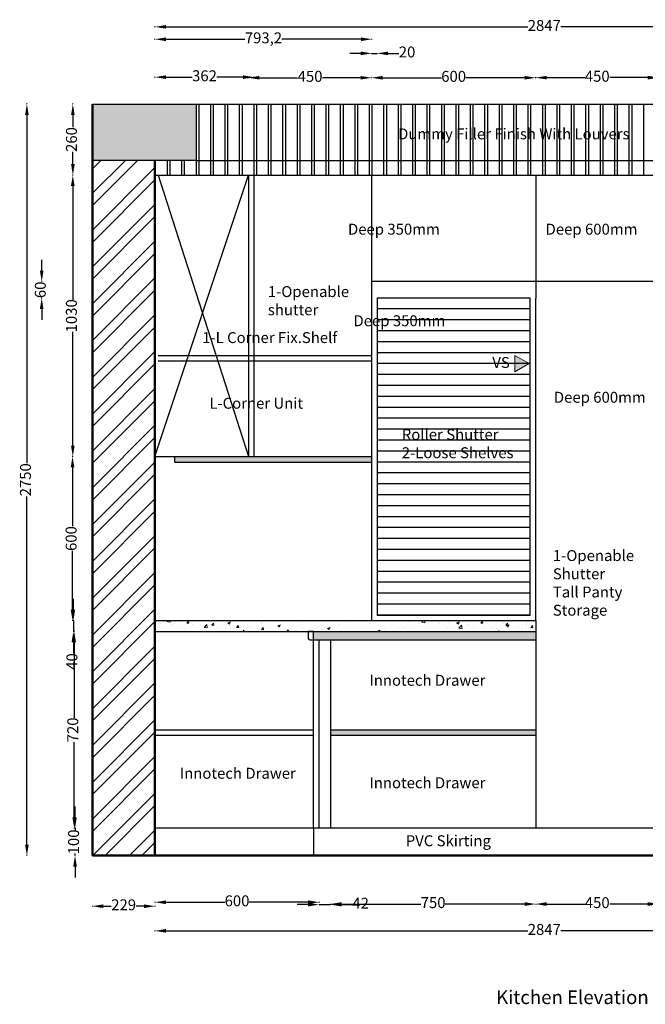
# Model space of a CAD drawing. Units: millimetres. Extents: x 2054 to 5837, y -782 to 2821.
# Tile 1 of 2: x 2054 to 4342, y -782 to 2821. Entities that reach past the tile are written whole.
import ezdxf

# ---------------------------------------------------------------- set-up
doc = ezdxf.new("R2010")
doc.units = ezdxf.units.MM
for name, color, linetype, lineweight in [('A-ANNO-DIMS', 2, 'Continuous', 18), ('A-ANNO-SYMB', 1, 'Continuous', 18), ('A-ANNO-TEXT', 7, 'Continuous', 18), ('A-FURN', 42, 'Continuous', 25), ('A-FURN-PATT', 8, 'Continuous', 13), ('A-WALL', 7, 'Continuous', 50), ('A-WALL-PATT', 8, 'Continuous', 13)]:
    doc.layers.add(name, color=color, linetype=linetype, lineweight=lineweight)
doc.styles.get("Standard").update_dxf_attribs({"font": 'arial.ttf'})
doc.dimstyles.new('ISO-25', dxfattribs={"dimtxt": 40, "dimasz": 40, "dimexe": 1.25, "dimexo": 0.625, "dimtad": 0, "dimtxsty": 'Standard', "dimcen": 2.5, "dimclrt": 1, "dimadec": 0, "dimazin": 0, "dimtfac": 1, "dimtmove": 0, "dimatfit": 3, "dimfxl": 1, "dimfxlon": 1, "dimarcsym": 0})

# ---------------------------------------------------------------- blocks, each defined once
blk = doc.blocks.new('*D2')
at = {"layer": 'A-ANNO-DIMS', "color": 0, "lineweight": -2, "transparency": 16777216}
for p, q in [((3941.1, -414.1), (3941.1, -416.4)), ((3981.1, -415.1), (4120.6, -415.1)), ((4351.1, -415.1), (4211.7, -415.1)), ((4391.1, -414.1), (4391.1, -416.4))]:
    blk.add_line(p, q, dxfattribs=at)
at = {"layer": 'A-ANNO-DIMS', "color": 0, "transparency": 16777216}
for points in [[(3981.1, -408.4), (3981.1, -421.8), (3941.1, -415.1)], [(4351.1, -408.4), (4351.1, -421.8), (4391.1, -415.1)]]:
    blk.add_solid(points, dxfattribs=at)
at = {"layer": 'Defpoints', "color": 0, "transparency": 16777216}
for p in [(3941.1, -137.8), (4391.1, -137.8), (3941.1, -415.1)]:
    blk.add_point(p, dxfattribs=at)
at = {"layer": 'A-ANNO-DIMS', "color": 0, "transparency": 16777216, "insert": (4166.1, -415.1), "char_height": 40, "attachment_point": 5}
blk.add_mtext('450', dxfattribs=at)
blk = doc.blocks.new('*D3')
at = {"layer": 'A-ANNO-DIMS', "color": 0, "lineweight": -2, "transparency": 16777216}
for p, q in [((3191.1, -414.1), (3191.1, -416.4)), ((3231.1, -415.1), (3521.5, -415.1)), ((3901.1, -415.1), (3610.7, -415.1)), ((3941.1, -414.1), (3941.1, -416.4))]:
    blk.add_line(p, q, dxfattribs=at)
at = {"layer": 'A-ANNO-DIMS', "color": 0, "transparency": 16777216}
for points in [[(3231.1, -408.4), (3231.1, -421.8), (3191.1, -415.1)], [(3901.1, -408.4), (3901.1, -421.8), (3941.1, -415.1)]]:
    blk.add_solid(points, dxfattribs=at)
at = {"layer": 'Defpoints', "color": 0, "transparency": 16777216}
for p in [(3191.1, -137.8), (3941.1, -137.8), (3191.1, -415.1)]:
    blk.add_point(p, dxfattribs=at)
at = {"layer": 'A-ANNO-DIMS', "color": 0, "transparency": 16777216, "insert": (3566.1, -415.1), "char_height": 40, "attachment_point": 5}
blk.add_mtext('750', dxfattribs=at)
blk = doc.blocks.new('*D4')
at = {"layer": 'A-ANNO-DIMS', "color": 0, "lineweight": -2, "transparency": 16777216}
for p, q in [((3109.1, -417.2), (3069.1, -417.2)), ((3149.1, -416.2), (3149.1, -418.5)), ((3149.1, -417.2), (3191.1, -417.2)), ((3191.1, -416.2), (3191.1, -418.5)), ((3231.1, -417.2), (3271.1, -417.2))]:
    blk.add_line(p, q, dxfattribs=at)
at = {"layer": 'A-ANNO-DIMS', "color": 0, "transparency": 16777216}
for points in [[(3109.1, -410.6), (3109.1, -423.9), (3149.1, -417.2)], [(3231.1, -410.6), (3231.1, -423.9), (3191.1, -417.2)]]:
    blk.add_solid(points, dxfattribs=at)
at = {"layer": 'Defpoints', "color": 0, "transparency": 16777216}
for p in [(3149.1, -137.8), (3191.1, -137.8), (3191.1, -417.2)]:
    blk.add_point(p, dxfattribs=at)
at = {"layer": 'A-ANNO-DIMS', "color": 0, "transparency": 16777216, "insert": (3301, -417.2), "char_height": 40, "attachment_point": 5}
blk.add_mtext('42', dxfattribs=at)
blk = doc.blocks.new('*D5')
at = {"layer": 'A-ANNO-DIMS', "color": 0, "lineweight": -2, "transparency": 16777216}
for p, q in [((2549.1, -407.6), (2549.1, -409.8)), ((2589.1, -408.6), (2804.3, -408.6)), ((3109.1, -408.6), (2894, -408.6)), ((3149.1, -407.6), (3149.1, -409.8))]:
    blk.add_line(p, q, dxfattribs=at)
at = {"layer": 'A-ANNO-DIMS', "color": 0, "transparency": 16777216}
for points in [[(2589.1, -401.9), (2589.1, -415.3), (2549.1, -408.6)], [(3109.1, -401.9), (3109.1, -415.3), (3149.1, -408.6)]]:
    blk.add_solid(points, dxfattribs=at)
at = {"layer": 'Defpoints', "color": 0, "transparency": 16777216}
for p in [(2549.1, -137.8), (3149.1, -137.8), (2549.1, -408.6)]:
    blk.add_point(p, dxfattribs=at)
at = {"layer": 'A-ANNO-DIMS', "color": 0, "transparency": 16777216, "insert": (2849.1, -408.6), "char_height": 40, "attachment_point": 5}
blk.add_mtext('600', dxfattribs=at)
blk = doc.blocks.new('*D6')
at = {"layer": 'A-ANNO-DIMS', "color": 0, "lineweight": -2, "transparency": 16777216}
for p, q in [((2549.1, -512.1), (2549.1, -514.3)), ((2589.1, -513.1), (3911.9, -513.1)), ((5356.1, -513.1), (4033.3, -513.1)), ((5396.1, -512.1), (5396.1, -514.3))]:
    blk.add_line(p, q, dxfattribs=at)
at = {"layer": 'A-ANNO-DIMS', "color": 0, "transparency": 16777216}
for points in [[(2589.1, -506.4), (2589.1, -519.7), (2549.1, -513.1)], [(5356.1, -506.4), (5356.1, -519.7), (5396.1, -513.1)]]:
    blk.add_solid(points, dxfattribs=at)
at = {"layer": 'Defpoints', "color": 0, "transparency": 16777216}
for p in [(2549.1, -237.8), (5396.1, -237.8), (5396.1, -513.1)]:
    blk.add_point(p, dxfattribs=at)
at = {"layer": 'A-ANNO-DIMS', "color": 0, "transparency": 16777216, "insert": (3972.6, -513.1), "char_height": 40, "attachment_point": 5}
blk.add_mtext('2847', dxfattribs=at)
blk = doc.blocks.new('*D13')
at = {"layer": 'A-ANNO-DIMS', "color": 0, "lineweight": -2, "transparency": 16777216}
for p, q in [((3941.1, 2607.6), (3941.1, 2609.9)), ((3981.1, 2608.6), (4120.6, 2608.6)), ((4351.1, 2608.6), (4211.7, 2608.6)), ((4391.1, 2607.6), (4391.1, 2609.9))]:
    blk.add_line(p, q, dxfattribs=at)
at = {"layer": 'A-ANNO-DIMS', "color": 0, "transparency": 16777216}
for points in [[(3981.1, 2615.3), (3981.1, 2602), (3941.1, 2608.6)], [(4351.1, 2615.3), (4351.1, 2602), (4391.1, 2608.6)]]:
    blk.add_solid(points, dxfattribs=at)
at = {"layer": 'Defpoints', "color": 0, "transparency": 16777216}
for p in [(3941.1, 2608.6), (3941.1, 2252.2), (4391.1, 2252.2)]:
    blk.add_point(p, dxfattribs=at)
at = {"layer": 'A-ANNO-DIMS', "color": 0, "transparency": 16777216, "insert": (4166.1, 2608.6), "char_height": 40, "attachment_point": 5}
blk.add_mtext('450', dxfattribs=at)
blk = doc.blocks.new('*D14')
at = {"layer": 'A-ANNO-DIMS', "color": 0, "lineweight": -2, "transparency": 16777216}
for p, q in [((3341.1, 2607.2), (3341.1, 2609.5)), ((3381.1, 2608.2), (3596.3, 2608.2)), ((3901.1, 2608.2), (3686, 2608.2)), ((3941.1, 2607.2), (3941.1, 2609.5))]:
    blk.add_line(p, q, dxfattribs=at)
at = {"layer": 'A-ANNO-DIMS', "color": 0, "transparency": 16777216}
for points in [[(3381.1, 2614.9), (3381.1, 2601.6), (3341.1, 2608.2)], [(3901.1, 2614.9), (3901.1, 2601.6), (3941.1, 2608.2)]]:
    blk.add_solid(points, dxfattribs=at)
at = {"layer": 'Defpoints', "color": 0, "transparency": 16777216}
for p in [(3341.1, 2608.2), (3341.1, 2252.2), (3941.1, 2252.2)]:
    blk.add_point(p, dxfattribs=at)
at = {"layer": 'A-ANNO-DIMS', "color": 0, "transparency": 16777216, "insert": (3641.1, 2608.2), "char_height": 40, "attachment_point": 5}
blk.add_mtext('600', dxfattribs=at)
blk = doc.blocks.new('*D15')
at = {"layer": 'A-ANNO-DIMS', "color": 0, "lineweight": -2, "transparency": 16777216}
for p, q in [((2891.1, 2607.2), (2891.1, 2609.5)), ((2931.1, 2608.2), (3070.6, 2608.2)), ((3301.1, 2608.2), (3161.7, 2608.2)), ((3341.1, 2607.2), (3341.1, 2609.5))]:
    blk.add_line(p, q, dxfattribs=at)
at = {"layer": 'A-ANNO-DIMS', "color": 0, "transparency": 16777216}
for points in [[(2931.1, 2614.9), (2931.1, 2601.6), (2891.1, 2608.2)], [(3301.1, 2614.9), (3301.1, 2601.6), (3341.1, 2608.2)]]:
    blk.add_solid(points, dxfattribs=at)
at = {"layer": 'Defpoints', "color": 0, "transparency": 16777216}
for p in [(3341.1, 2608.2), (2891.1, 2252.2), (3341.1, 2252.2)]:
    blk.add_point(p, dxfattribs=at)
at = {"layer": 'A-ANNO-DIMS', "color": 0, "transparency": 16777216, "insert": (3116.1, 2608.2), "char_height": 40, "attachment_point": 5}
blk.add_mtext('450', dxfattribs=at)
blk = doc.blocks.new('*D16')
at = {"layer": 'A-ANNO-DIMS', "color": 0, "lineweight": -2, "transparency": 16777216}
for p, q in [((2549.1, 2609.3), (2549.1, 2611.6)), ((2589.1, 2610.3), (2685.5, 2610.3)), ((2871.1, 2610.3), (2774.7, 2610.3)), ((2911.1, 2609.3), (2911.1, 2611.6))]:
    blk.add_line(p, q, dxfattribs=at)
at = {"layer": 'A-ANNO-DIMS', "color": 0, "transparency": 16777216}
for points in [[(2589.1, 2617), (2589.1, 2603.7), (2549.1, 2610.3)], [(2871.1, 2617), (2871.1, 2603.7), (2911.1, 2610.3)]]:
    blk.add_solid(points, dxfattribs=at)
at = {"layer": 'Defpoints', "color": 0, "transparency": 16777216}
for p in [(2549.1, 2610.3), (2549.1, 2252.2), (2911.1, 2252.2)]:
    blk.add_point(p, dxfattribs=at)
at = {"layer": 'A-ANNO-DIMS', "color": 0, "transparency": 16777216, "insert": (2730.1, 2610.3), "char_height": 40, "attachment_point": 5}
blk.add_mtext('362', dxfattribs=at)
blk = doc.blocks.new('*D17')
at = {"layer": 'A-ANNO-DIMS', "color": 0, "lineweight": -2, "transparency": 16777216}
for p, q in [((2549.1, 2748.1), (2549.1, 2750.3)), ((2589.1, 2749.1), (2878, 2749.1)), ((3302.3, 2749.1), (3013.5, 2749.1)), ((3342.3, 2748.1), (3342.3, 2750.3))]:
    blk.add_line(p, q, dxfattribs=at)
at = {"layer": 'A-ANNO-DIMS', "color": 0, "transparency": 16777216}
for points in [[(2589.1, 2755.7), (2589.1, 2742.4), (2549.1, 2749.1)], [(3302.3, 2755.7), (3302.3, 2742.4), (3342.3, 2749.1)]]:
    blk.add_solid(points, dxfattribs=at)
at = {"layer": 'Defpoints', "color": 0, "transparency": 16777216}
for p in [(2549.1, 2749.1), (2549.1, 2252.2), (3342.3, 2252.2)]:
    blk.add_point(p, dxfattribs=at)
at = {"layer": 'A-ANNO-DIMS', "color": 0, "transparency": 16777216, "insert": (2945.7, 2749.1), "char_height": 40, "attachment_point": 5}
blk.add_mtext('793,2', dxfattribs=at)
blk = doc.blocks.new('*D18')
at = {"layer": 'A-ANNO-DIMS', "color": 0, "lineweight": -2, "transparency": 16777216}
for p, q in [((2549.1, 2793.4), (2549.1, 2795.7)), ((2589.1, 2794.4), (3911.9, 2794.4)), ((5356.1, 2794.4), (4033.3, 2794.4)), ((5396.1, 2793.4), (5396.1, 2795.7))]:
    blk.add_line(p, q, dxfattribs=at)
at = {"layer": 'A-ANNO-DIMS', "color": 0, "transparency": 16777216}
for points in [[(2589.1, 2801.1), (2589.1, 2787.8), (2549.1, 2794.4)], [(5356.1, 2801.1), (5356.1, 2787.8), (5396.1, 2794.4)]]:
    blk.add_solid(points, dxfattribs=at)
at = {"layer": 'Defpoints', "color": 0, "transparency": 16777216}
for p in [(5396.1, 2794.4), (2549.1, 2306), (5396.1, 2252.2)]:
    blk.add_point(p, dxfattribs=at)
at = {"layer": 'A-ANNO-DIMS', "color": 0, "transparency": 16777216, "insert": (3972.6, 2794.4), "char_height": 40, "attachment_point": 5}
blk.add_mtext('2847', dxfattribs=at)
blk = doc.blocks.new('*D19')
at = {"layer": 'A-ANNO-DIMS', "color": 0, "lineweight": -2, "transparency": 16777216}
for p, q in [((2249.8, 2512.2), (2247.6, 2512.2)), ((2248.8, 2472.2), (2248.8, 2427.3)), ((2248.8, 2292.2), (2248.8, 2337.1)), ((2249.8, 2252.2), (2247.6, 2252.2))]:
    blk.add_line(p, q, dxfattribs=at)
at = {"layer": 'A-ANNO-DIMS', "color": 0, "transparency": 16777216}
for points in [[(2242.2, 2472.2), (2255.5, 2472.2), (2248.8, 2512.2)], [(2242.2, 2292.2), (2255.5, 2292.2), (2248.8, 2252.2)]]:
    blk.add_solid(points, dxfattribs=at)
at = {"layer": 'Defpoints', "color": 0, "transparency": 16777216}
for p in [(2248.8, 2512.2), (2549.1, 2512.2), (2549.1, 2252.2)]:
    blk.add_point(p, dxfattribs=at)
at = {"layer": 'A-ANNO-DIMS', "color": 0, "transparency": 16777216, "insert": (2248.8, 2382.2), "char_height": 40, "attachment_point": 5, "rotation": 90}
blk.add_mtext('260', dxfattribs=at)
blk = doc.blocks.new('*D20')
at = {"layer": 'A-ANNO-DIMS', "color": 0, "lineweight": -2, "transparency": 16777216}
for p, q in [((2249.6, 2252.2), (2247.3, 2252.2)), ((2248.6, 2212.2), (2248.6, 1795.6)), ((2248.6, 1262.2), (2248.6, 1678.8)), ((2249.6, 1222.2), (2247.3, 1222.2))]:
    blk.add_line(p, q, dxfattribs=at)
at = {"layer": 'A-ANNO-DIMS', "color": 0, "transparency": 16777216}
for points in [[(2241.9, 2212.2), (2255.2, 2212.2), (2248.6, 2252.2)], [(2241.9, 1262.2), (2255.2, 1262.2), (2248.6, 1222.2)]]:
    blk.add_solid(points, dxfattribs=at)
at = {"layer": 'Defpoints', "color": 0, "transparency": 16777216}
for p in [(2549.1, 2252.2), (2248.6, 1222.2), (2549.1, 1222.2)]:
    blk.add_point(p, dxfattribs=at)
at = {"layer": 'A-ANNO-DIMS', "color": 0, "transparency": 16777216, "insert": (2248.6, 1737.2), "char_height": 40, "attachment_point": 5, "rotation": 90}
blk.add_mtext('1030', dxfattribs=at)
blk = doc.blocks.new('*D21')
at = {"layer": 'A-ANNO-DIMS', "color": 0, "lineweight": -2, "transparency": 16777216}
for p, q in [((2248.6, 1222.2), (2246.4, 1222.2)), ((2247.6, 1182.2), (2247.6, 967)), ((2247.6, 662.2), (2247.6, 877.3)), ((2248.6, 622.2), (2246.4, 622.2))]:
    blk.add_line(p, q, dxfattribs=at)
at = {"layer": 'A-ANNO-DIMS', "color": 0, "transparency": 16777216}
for points in [[(2240.9, 1182.2), (2254.3, 1182.2), (2247.6, 1222.2)], [(2240.9, 662.2), (2254.3, 662.2), (2247.6, 622.2)]]:
    blk.add_solid(points, dxfattribs=at)
at = {"layer": 'Defpoints', "color": 0, "transparency": 16777216}
for p in [(2549.1, 1222.2), (2247.6, 622.2), (2549.1, 622.2)]:
    blk.add_point(p, dxfattribs=at)
at = {"layer": 'A-ANNO-DIMS', "color": 0, "transparency": 16777216, "insert": (2247.6, 922.2), "char_height": 40, "attachment_point": 5, "rotation": 90}
blk.add_mtext('600', dxfattribs=at)
blk = doc.blocks.new('*D22')
at = {"layer": 'A-ANNO-DIMS', "color": 0, "lineweight": -2, "transparency": 16777216}
for p, q in [((2250.6, 662.2), (2250.6, 702.2)), ((2251.6, 622.2), (2249.4, 622.2)), ((2250.6, 622.2), (2250.6, 582.2)), ((2251.6, 582.2), (2249.4, 582.2)), ((2250.6, 542.2), (2250.6, 502.2))]:
    blk.add_line(p, q, dxfattribs=at)
at = {"layer": 'A-ANNO-DIMS', "color": 0, "transparency": 16777216}
for points in [[(2244, 662.2), (2257.3, 662.2), (2250.6, 622.2)], [(2244, 542.2), (2257.3, 542.2), (2250.6, 582.2)]]:
    blk.add_solid(points, dxfattribs=at)
at = {"layer": 'Defpoints', "color": 0, "transparency": 16777216}
for p in [(2549.1, 622.2), (2250.6, 582.2), (2549.1, 582.2)]:
    blk.add_point(p, dxfattribs=at)
at = {"layer": 'A-ANNO-DIMS', "color": 0, "transparency": 16777216, "insert": (2250.6, 472.2), "char_height": 40, "attachment_point": 5, "rotation": 90}
blk.add_mtext('40', dxfattribs=at)
blk = doc.blocks.new('*D23')
at = {"layer": 'A-ANNO-DIMS', "color": 0, "lineweight": -2, "transparency": 16777216}
for p, q in [((2254.7, 582.2), (2252.4, 582.2)), ((2253.7, 542.2), (2253.7, 266.8)), ((2253.7, -97.8), (2253.7, 177.6)), ((2254.7, -137.8), (2252.4, -137.8))]:
    blk.add_line(p, q, dxfattribs=at)
at = {"layer": 'A-ANNO-DIMS', "color": 0, "transparency": 16777216}
for points in [[(2247, 542.2), (2260.3, 542.2), (2253.7, 582.2)], [(2247, -97.8), (2260.3, -97.8), (2253.7, -137.8)]]:
    blk.add_solid(points, dxfattribs=at)
at = {"layer": 'Defpoints', "color": 0, "transparency": 16777216}
for p in [(2549.1, 582.2), (2253.7, -137.8), (2549.1, -137.8)]:
    blk.add_point(p, dxfattribs=at)
at = {"layer": 'A-ANNO-DIMS', "color": 0, "transparency": 16777216, "insert": (2253.7, 222.2), "char_height": 40, "attachment_point": 5, "rotation": 90}
blk.add_mtext('720', dxfattribs=at)
blk = doc.blocks.new('*D24')
at = {"layer": 'A-ANNO-DIMS', "color": 0, "lineweight": -2, "transparency": 16777216}
for p, q in [((2256.7, -97.8), (2256.7, -57.8)), ((2257.7, -137.8), (2255.5, -137.8)), ((2256.7, -137.8), (2256.7, -144.9)), ((2257.7, -237.8), (2255.5, -237.8)), ((2256.7, -237.8), (2256.7, -230.7)), ((2256.7, -277.8), (2256.7, -317.8))]:
    blk.add_line(p, q, dxfattribs=at)
at = {"layer": 'A-ANNO-DIMS', "color": 0, "transparency": 16777216}
for points in [[(2250, -97.8), (2263.4, -97.8), (2256.7, -137.8)], [(2250, -277.8), (2263.4, -277.8), (2256.7, -237.8)]]:
    blk.add_solid(points, dxfattribs=at)
at = {"layer": 'Defpoints', "color": 0, "transparency": 16777216}
for p in [(2549.1, -137.8), (2256.7, -237.8), (2549.1, -237.8)]:
    blk.add_point(p, dxfattribs=at)
at = {"layer": 'A-ANNO-DIMS', "color": 0, "transparency": 16777216, "insert": (2256.7, -187.8), "char_height": 40, "attachment_point": 5, "rotation": 90}
blk.add_mtext('100', dxfattribs=at)
blk = doc.blocks.new('*D25')
at = {"layer": 'A-ANNO-DIMS', "color": 0, "lineweight": -2, "transparency": 16777216}
for p, q in [((2081.7, 2512.2), (2079.4, 2512.2)), ((2080.7, 2472.2), (2080.7, 1197.8)), ((2080.7, -197.8), (2080.7, 1076.6)), ((2081.7, -237.8), (2079.4, -237.8))]:
    blk.add_line(p, q, dxfattribs=at)
at = {"layer": 'A-ANNO-DIMS', "color": 0, "transparency": 16777216}
for points in [[(2074, 2472.2), (2087.4, 2472.2), (2080.7, 2512.2)], [(2074, -197.8), (2087.4, -197.8), (2080.7, -237.8)]]:
    blk.add_solid(points, dxfattribs=at)
at = {"layer": 'Defpoints', "color": 0, "transparency": 16777216}
for p in [(2320.1, 2512.2), (2080.7, -237.8), (2320.1, -237.8)]:
    blk.add_point(p, dxfattribs=at)
at = {"layer": 'A-ANNO-DIMS', "color": 0, "transparency": 16777216, "insert": (2080.7, 1137.2), "char_height": 40, "attachment_point": 5, "rotation": 90}
blk.add_mtext('2750', dxfattribs=at)
blk = doc.blocks.new('VS-MARKER')
h = blk.add_hatch(color=256)
h.dxf.hatch_style = 1
h.paths.add_polyline_path([(0, 0), (60, 0), (30, 52)])
blk.add_lwpolyline([(0, 0), (60, 0), (30, 52), (0, 0)])
blk = doc.blocks.new('*D30')
at = {"layer": 'A-ANNO-DIMS', "color": 0, "lineweight": -2, "transparency": 16777216}
for p, q in [((2320.1, -422.1), (2320.1, -424.3)), ((2360.1, -423.1), (2389.4, -423.1)), ((2509.1, -423.1), (2479.8, -423.1)), ((2549.1, -422.1), (2549.1, -424.3))]:
    blk.add_line(p, q, dxfattribs=at)
at = {"layer": 'A-ANNO-DIMS', "color": 0, "transparency": 16777216}
for points in [[(2360.1, -416.4), (2360.1, -429.7), (2320.1, -423.1)], [(2509.1, -416.4), (2509.1, -429.7), (2549.1, -423.1)]]:
    blk.add_solid(points, dxfattribs=at)
at = {"layer": 'Defpoints', "color": 0, "transparency": 16777216}
for p in [(2320.1, -237.8), (2549.1, -237.8), (2549.1, -423.1)]:
    blk.add_point(p, dxfattribs=at)
at = {"layer": 'A-ANNO-DIMS', "color": 1, "transparency": 16777216, "insert": (2434.6, -423.1), "char_height": 40, "attachment_point": 5}
blk.add_mtext('229', dxfattribs=at)
blk = doc.blocks.new('*D32')
at = {"layer": 'A-ANNO-DIMS', "color": 0, "lineweight": -2, "transparency": 16777216}
for p, q in [((5809.4, 1802.2), (5811.6, 1802.2)), ((5810.4, 1762.2), (5810.4, 1280.6)), ((5810.4, 682.2), (5810.4, 1163.8)), ((5809.4, 642.2), (5811.6, 642.2))]:
    blk.add_line(p, q, dxfattribs=at)
at = {"layer": 'A-ANNO-DIMS', "color": 0, "transparency": 16777216}
for points in [[(5803.7, 1762.2), (5817, 1762.2), (5810.4, 1802.2)], [(5803.7, 682.2), (5817, 682.2), (5810.4, 642.2)]]:
    blk.add_solid(points, dxfattribs=at)
at = {"layer": 'Defpoints', "color": 0, "transparency": 16777216}
for p in [(3921.1, 1802.2), (5810.4, 1802.2), (3921.1, 642.2)]:
    blk.add_point(p, dxfattribs=at)
at = {"layer": 'A-ANNO-DIMS', "color": 1, "transparency": 16777216, "insert": (5810.4, 1222.2), "char_height": 40, "attachment_point": 5, "rotation": 90}
blk.add_mtext('1160', dxfattribs=at)
blk = doc.blocks.new('*D33')
at = {"layer": 'A-ANNO-DIMS', "color": 0, "lineweight": -2, "transparency": 16777216}
for p, q in [((3301.1, 2697.4), (3261.1, 2697.4)), ((3341.1, 2696.4), (3341.1, 2698.7)), ((3341.1, 2697.4), (3361.1, 2697.4)), ((3361.1, 2696.4), (3361.1, 2698.7)), ((3401.1, 2697.4), (3441.1, 2697.4))]:
    blk.add_line(p, q, dxfattribs=at)
at = {"layer": 'A-ANNO-DIMS', "color": 0, "transparency": 16777216}
for points in [[(3301.1, 2704.1), (3301.1, 2690.8), (3341.1, 2697.4)], [(3401.1, 2704.1), (3401.1, 2690.8), (3361.1, 2697.4)]]:
    blk.add_solid(points, dxfattribs=at)
at = {"layer": 'Defpoints', "color": 0, "transparency": 16777216}
for p in [(3361.1, 2697.4), (3341.1, 1802.2), (3361.1, 1802.2)]:
    blk.add_point(p, dxfattribs=at)
at = {"layer": 'A-ANNO-DIMS', "color": 1, "transparency": 16777216, "insert": (3470.7, 2697.4), "char_height": 40, "attachment_point": 5}
blk.add_mtext('20', dxfattribs=at)
blk = doc.blocks.new('*D34')
at = {"layer": 'A-ANNO-DIMS', "color": 0, "lineweight": -2, "transparency": 16777216}
for p, q in [((2134.9, 1902.2), (2134.9, 1942.2)), ((2135.9, 1862.2), (2133.6, 1862.2)), ((2134.9, 1862.2), (2134.9, 1861.5)), ((2135.9, 1802.2), (2133.6, 1802.2)), ((2134.9, 1802.2), (2134.9, 1802.9)), ((2134.9, 1762.2), (2134.9, 1722.2))]:
    blk.add_line(p, q, dxfattribs=at)
at = {"layer": 'A-ANNO-DIMS', "color": 0, "transparency": 16777216}
for points in [[(2128.2, 1902.2), (2141.5, 1902.2), (2134.9, 1862.2)], [(2128.2, 1762.2), (2141.5, 1762.2), (2134.9, 1802.2)]]:
    blk.add_solid(points, dxfattribs=at)
at = {"layer": 'Defpoints', "color": 0, "transparency": 16777216}
for p in [(2134.9, 1862.2), (3341.1, 1862.2), (3361.1, 1802.2)]:
    blk.add_point(p, dxfattribs=at)
at = {"layer": 'A-ANNO-DIMS', "color": 1, "transparency": 16777216, "insert": (2134.9, 1832.2), "char_height": 40, "attachment_point": 5, "rotation": 90}
blk.add_mtext('60', dxfattribs=at)

msp = doc.modelspace()

# ---------------------------------------------------------------- hatches: boundary and pattern name
at = {"layer": 'A-FURN-PATT'}
h = msp.add_hatch(dxfattribs=at)
h.set_pattern_fill('AR-CONC', color=256, scale=0.5)
h.paths.add_polyline_path([(2699.109, 2512.19), (2320.109, 2512.19), (2320.109, 2306.028), (2699.109, 2306.028)])
h.paths.add_polyline_path([(5625.109, 2512.19), (5310.109, 2512.19), (5310.109, 2252.19), (5625.109, 2252.19)])
h = msp.add_hatch(color=256, dxfattribs=at)
h.dxf.hatch_style = 1
h.paths.add_polyline_path([(3341.109, 1222.19), (2622.052, 1222.19), (2622.052, 1202.19), (3341.109, 1202.19)])
h = msp.add_hatch(dxfattribs=at)
h.set_pattern_fill('AR-CONC', color=256, scale=0.5)
h.paths.add_polyline_path([(3941.109, 622.19), (3341.109, 622.19), (2549.109, 622.19), (2549.109, 582.19), (3129.109, 582.19), (3941.109, 582.19)])
h = msp.add_hatch(color=256, dxfattribs=at)
h.dxf.hatch_style = 1
h.paths.add_polyline_path([(3941.109, 552.19), (3941.109, 582.19), (3129.109, 582.19), (3129.109, 552.19)])
h.paths.add_polyline_path([(3941.109, 202.19), (3941.109, 222.19), (3191.109, 222.19), (3191.109, 202.19)])
at = {"layer": 'A-WALL-PATT'}
h = msp.add_hatch(dxfattribs=at)
h.set_pattern_fill('ANSI32', color=256, scale=10)
h.paths.add_polyline_path([(2549.109, 2306.028), (2320.109, 2306.028), (2320.109, -237.81), (2549.109, -237.81), (2549.109, 582.19), (2549.109, 622.19), (2549.109, 1222.19)])
h.paths.add_polyline_path([(5625.109, 2252.19), (5396.109, 2252.19), (5396.109, 1862.19), (5396.109, -237.81), (5625.109, -237.81)])

# ---------------------------------------------------------------- linework, layer by layer
at = {"layer": 'A-FURN'}
for p, q in [((2320.109, 2512.19), (2699.109, 2512.19)), ((2699.109, 2512.19), (2699.109, 2306.028)), ((2699.109, 2512.19), (5310.109, 2512.19)), ((2699.109, 2512.19), (2699.109, 2306.028)), ((2709.109, 2512.19), (2709.109, 2252.19)), ((2751.876, 2512.19), (2751.876, 2252.19)), ((2761.876, 2512.19), (2761.876, 2252.19)), ((2804.643, 2512.19), (2804.643, 2252.19)), ((2814.643, 2512.19), (2814.643, 2252.19)), ((2857.41, 2512.19), (2857.41, 2252.19)), ((2867.41, 2512.19), (2867.41, 2252.19)), ((2910.177, 2512.19), (2910.177, 2252.19)), ((2920.177, 2512.19), (2920.177, 2252.19)), ((2962.944, 2512.19), (2962.944, 2252.19)), ((2972.944, 2512.19), (2972.944, 2252.19)), ((3015.71, 2512.19), (3015.71, 2252.19)), ((3025.71, 2512.19), (3025.71, 2252.19)), ((3068.477, 2512.19), (3068.477, 2252.19)), ((3078.477, 2512.19), (3078.477, 2252.19)), ((3121.244, 2512.19), (3121.244, 2252.19)), ((3131.244, 2512.19), (3131.244, 2252.19)), ((3174.011, 2512.19), (3174.011, 2252.19)), ((3184.011, 2512.19), (3184.011, 2252.19)), ((3226.778, 2512.19), (3226.778, 2252.19)), ((3236.778, 2512.19), (3236.778, 2252.19)), ((3279.545, 2512.19), (3279.545, 2252.19)), ((3289.545, 2512.19), (3289.545, 2252.19)), ((3332.312, 2512.19), (3332.312, 2252.19)), ((3342.312, 2512.19), (3342.312, 2252.19)), ((3385.078, 2512.19), (3385.078, 2252.19)), ((3395.078, 2512.19), (3395.078, 2252.19)), ((3437.845, 2512.19), (3437.845, 2252.19)), ((3447.845, 2512.19), (3447.845, 2252.19)), ((3490.612, 2512.19), (3490.612, 2252.19)), ((3500.612, 2512.19), (3500.612, 2252.19)), ((3543.379, 2512.19), (3543.379, 2252.19)), ((3553.379, 2512.19), (3553.379, 2252.19)), ((3596.146, 2512.19), (3596.146, 2252.19)), ((3606.146, 2512.19), (3606.146, 2252.19)), ((3648.913, 2512.19), (3648.913, 2252.19)), ((3658.913, 2512.19), (3658.913, 2252.19)), ((3701.679, 2512.19), (3701.679, 2252.19)), ((3711.679, 2512.19), (3711.679, 2252.19)), ((3754.446, 2512.19), (3754.446, 2252.19)), ((3764.446, 2512.19), (3764.446, 2252.19)), ((3807.213, 2512.19), (3807.213, 2252.19)), ((3817.213, 2512.19), (3817.213, 2252.19)), ((3859.98, 2512.19), (3859.98, 2252.19)), ((3869.98, 2512.19), (3869.98, 2252.19)), ((3912.747, 2512.19), (3912.747, 2252.19)), ((3922.747, 2512.19), (3922.747, 2252.19)), ((3965.514, 2512.19), (3965.514, 2252.19)), ((3975.514, 2512.19), (3975.514, 2252.19)), ((4018.281, 2512.19), (4018.281, 2252.19)), ((4028.281, 2512.19), (4028.281, 2252.19)), ((4071.047, 2512.19), (4071.047, 2252.19)), ((4081.047, 2512.19), (4081.047, 2252.19)), ((4123.814, 2512.19), (4123.814, 2252.19)), ((4133.814, 2512.19), (4133.814, 2252.19)), ((4176.581, 2512.19), (4176.581, 2252.19)), ((4186.581, 2512.19), (4186.581, 2252.19)), ((4229.348, 2512.19), (4229.348, 2252.19)), ((4239.348, 2512.19), (4239.348, 2252.19)), ((4282.115, 2512.19), (4282.115, 2252.19)), ((4292.115, 2512.19), (4292.115, 2252.19)), ((4334.882, 2512.19), (4334.882, 2252.19)), ((2699.109, 2306.028), (2320.109, 2306.028)), ((2593.569, 2306.028), (2593.569, 2252.19)), ((2603.569, 2306.028), (2603.569, 2252.19)), ((2646.339, 2306.028), (2646.339, 2252.19)), ((2656.339, 2306.028), (2656.339, 2252.19)), ((2699.109, 2306.028), (2699.109, 2252.19)), ((2699.109, 2306.028), (5310.109, 2306.028)), ((2549.109, 2252.19), (5310.109, 2252.19)), ((2549.109, 1222.19), (2891.109, 2252.19)), ((2561.109, 2252.19), (2891.109, 1222.19)), ((2891.109, 2252.19), (2891.109, 1222.19)), ((2911.109, 2252.19), (2911.109, 1222.19)), ((3341.109, 2252.19), (3341.109, 1862.19)), ((3941.109, 2252.19), (3941.109, 1862.19)), ((3341.109, 1862.19), (3341.109, 1802.19)), ((3941.109, 1862.19), (3341.109, 1862.19)), ((5396.109, 1862.19), (3941.109, 1862.19)), ((3941.109, 1862.19), (3941.109, 1802.19)), ((3341.109, 1802.19), (3341.109, 622.19)), ((3361.109, 1802.19), (3361.109, 642.19)), ((3921.109, 1802.19), (3361.109, 1802.19)), ((3921.109, 642.19), (3921.109, 1802.19)), ((3941.109, 622.19), (3941.109, 1802.19)), ((3921.109, 1762.19), (3361.109, 1762.19)), ((3921.109, 1722.19), (3361.109, 1722.19)), ((3921.109, 1682.19), (3361.109, 1682.19)), ((3921.109, 1642.19), (3361.109, 1642.19)), ((2561.109, 1592.19), (3341.109, 1592.19)), ((3921.109, 1602.19), (3361.109, 1602.19)), ((2561.109, 1572.19), (3341.109, 1572.19)), ((3921.109, 1562.19), (3361.109, 1562.19)), ((3921.109, 1522.19), (3361.109, 1522.19)), ((3921.109, 1482.19), (3361.109, 1482.19)), ((3921.109, 1442.19), (3361.109, 1442.19)), ((3921.109, 1402.19), (3361.109, 1402.19)), ((3921.109, 1362.19), (3361.109, 1362.19)), ((3921.109, 1322.19), (3361.109, 1322.19)), ((3921.109, 1282.19), (3361.109, 1282.19)), ((3921.109, 1242.19), (3361.109, 1242.19)), ((2549.109, 1222.19), (3341.109, 1222.19)), ((2622.052, 1202.19), (2622.052, 1222.19)), ((2622.052, 1202.19), (3341.109, 1202.19)), ((3921.109, 1202.19), (3361.109, 1202.19)), ((3921.109, 1162.19), (3361.109, 1162.19)), ((3921.109, 1122.19), (3361.109, 1122.19)), ((3921.109, 1082.19), (3361.109, 1082.19)), ((3921.109, 1042.19), (3361.109, 1042.19)), ((3921.109, 1002.19), (3361.109, 1002.19)), ((3921.109, 962.19), (3361.109, 962.19)), ((3921.109, 922.19), (3361.109, 922.19)), ((3921.109, 882.19), (3361.109, 882.19)), ((3921.109, 842.19), (3361.109, 842.19)), ((3921.109, 802.19), (3361.109, 802.19)), ((3921.109, 762.19), (3361.109, 762.19)), ((3921.109, 722.19), (3361.109, 722.19)), ((3921.109, 682.19), (3361.109, 682.19)), ((2549.109, 622.19), (3341.109, 622.19)), ((3341.109, 622.19), (3941.109, 622.19)), ((3361.109, 642.19), (3921.109, 642.19)), ((3921.109, 642.19), (3361.109, 642.19)), ((3941.109, 622.19), (3941.109, 582.19)), ((2549.109, 582.19), (3129.109, 582.19)), ((3129.109, -137.81), (3129.109, 582.19)), ((3129.109, 582.19), (3941.109, 582.19)), ((3941.109, 582.19), (3941.109, -137.81)), ((3129.109, 552.19), (3941.109, 552.19)), ((3149.109, -137.81), (3149.109, 552.19)), ((3191.109, 552.19), (3191.109, -137.81)), ((2549.109, 222.19), (3129.109, 222.19)), ((3191.109, 222.19), (3941.109, 222.19)), ((2549.109, 202.19), (3129.109, 202.19)), ((3191.109, 202.19), (3941.109, 202.19)), ((5396.109, -137.81), (2549.109, -137.81)), ((3129.109, -137.81), (3129.109, -237.81))]:
    msp.add_line(p, q, dxfattribs=at)
msp.add_lwpolyline([(3129.109, 582.19), (3109.767, 582.19), (3109.767, 556.748, 0.41421356), (3114.767, 551.748), (3129.109, 551.748)], format="xyb", dxfattribs=at)
at = {"layer": 'A-WALL'}
for p, q in [((2320.109, 2306.028), (2320.109, 2512.19)), ((2320.109, -237.81), (2320.109, 2306.028)), ((2549.109, 1222.19), (2549.109, 2306.028)), ((2549.109, 622.19), (2549.109, 1222.19)), ((2549.109, 582.19), (2549.109, 622.19)), ((2549.109, -237.81), (2549.109, 582.19)), ((5625.109, -237.81), (2320.109, -237.81))]:
    msp.add_line(p, q, dxfattribs=at)

# ---------------------------------------------------------------- block references
at = {"layer": 'A-ANNO-SYMB', "rotation": 270.0000000000011}
msp.add_blockref('VS-MARKER', (3865.364, 1592.19), dxfattribs=at)

# ---------------------------------------------------------------- texts
at = {"layer": 'A-ANNO-SYMB', "attachment_point": 1}
for s, width, insert, char_height in [('VS', 129.91792, (3782.528, 1586.417), 40), ('{Kitchen Elevation At-C}', 1817.98967, (3796.43, -731.1), 50)]:
    msp.add_mtext_dynamic_manual_height_columns(s, width=width, gutter_width=12.5, heights=[0], dxfattribs=dict(at, insert=insert, char_height=char_height))
at = {"layer": 'A-ANNO-TEXT', "char_height": 40, "attachment_point": 1}
for s, width, insert in [('Dummy Filler Finish With Louvers', 972.79689, (3437.845, 2422.845)), ('{Deep 350mm}', 408.10443, (3254.765, 2074.157)), ('{Deep 600mm}', 408.10443, (3977.367, 2074.157)), ('1-Openable\\Pshutter', 505.9376, (2961.73, 1845.78)), ('{Deep 350mm}', 408.10443, (3274.765, 1739.157)), ('1-L Corner Fix.Shelf', 505.9376, (2721.653, 1677.473)), ('{Deep 600mm}', 408.10443, (4007.546, 1459.075)), ('L-Corner Unit', 505.9376, (2747.852, 1437.278)), ('Roller Shutter\\P2-Loose Shelves', 505.9376, (3451.563, 1322.845)), ('1-Openable\\PShutter\\PTall Panty\\PStorage', 505.9376, (4003.842, 879.957)), ('Innotech Drawer', 505.9376, (3333.098, 423.603)), ('Innotech Drawer', 505.9376, (2639.882, 83.307)), ('Innotech Drawer', 505.9376, (3333.098, 48.589)), ('PVC Skirting', 505.9376, (3466.063, -163.579))]:
    msp.add_mtext_dynamic_manual_height_columns(s, width=width, gutter_width=12.5, heights=[0], dxfattribs=dict(at, insert=insert))

# ---------------------------------------------------------------- dimensions: what is measured, and where the dimension line sits
at = {"layer": 'A-ANNO-DIMS'}
for base, p1, p2, override, picture, middle in [((5396.109, 2794.425), (2549.109, 2306.028), (5396.109, 2252.19), {"dimclrd": 0, "dimclre": 0, "dimclrt": 0}, '*D18', (3972.609, 2794.425)), ((2549.109, 2749.062), (3342.312, 2252.19), (2549.109, 2252.19), {"dimclrd": 0, "dimclre": 0, "dimclrt": 0}, '*D17', (2945.71, 2749.062)), ((3361.109, 2697.44), (3341.109, 1802.19), (3361.109, 1802.19), {"dimdec": 0, "dimlfac": 1, "dimrnd": 0, "dimzin": 0, "dimdsep": 46, "dimlunit": 2}, '*D33', (3470.657, 2697.44)), ((2549.109, 2610.333), (2911.109, 2252.19), (2549.109, 2252.19), {"dimclrd": 0, "dimclre": 0, "dimclrt": 0}, '*D16', (2730.109, 2610.333)), ((3341.109, 2608.242), (2891.109, 2252.19), (3341.109, 2252.19), {"dimclrd": 0, "dimclre": 0, "dimclrt": 0}, '*D15', (3116.109, 2608.242)), ((3341.109, 2608.242), (3941.109, 2252.19), (3341.109, 2252.19), {"dimclrd": 0, "dimclre": 0, "dimclrt": 0}, '*D14', (3641.109, 2608.242)), ((3941.109, 2608.643), (4391.109, 2252.19), (3941.109, 2252.19), {"dimclrd": 0, "dimclre": 0, "dimclrt": 0, "dimtmove": 1}, '*D13', (4166.109, 2608.643)), ((2549.109, -408.588), (3149.109, -137.81), (2549.109, -137.81), {"dimclrd": 0, "dimclre": 0, "dimclrt": 0}, '*D5', (2849.109, -408.588)), ((3191.109, -417.244), (3149.109, -137.81), (3191.109, -137.81), {"dimclrd": 0, "dimclre": 0, "dimclrt": 0}, '*D4', (3300.984, -417.244)), ((3191.109, -415.115), (3941.109, -137.81), (3191.109, -137.81), {"dimclrd": 0, "dimclre": 0, "dimclrt": 0, "dimtmove": 1}, '*D3', (3566.109, -415.115)), ((3941.109, -415.115), (4391.109, -137.81), (3941.109, -137.81), {"dimclrd": 0, "dimclre": 0, "dimclrt": 0, "dimtmove": 1}, '*D2', (4166.109, -415.115)), ((2549.109, -423.06), (2320.109, -237.81), (2549.109, -237.81), {"dimdec": 0, "dimlfac": 1, "dimrnd": 0, "dimzin": 0, "dimdsep": 46, "dimlunit": 2}, '*D30', (2434.609, -423.06)), ((5396.109, -513.067), (2549.109, -237.81), (5396.109, -237.81), {"dimclrd": 0, "dimclre": 0, "dimclrt": 0}, '*D6', (3972.609, -513.067))]:
    dim = msp.add_linear_dim(base=base, p1=p1, p2=p2, dimstyle='ISO-25', override=override, dxfattribs=at)
    dim.commit()
    dim.dimension.update_dxf_attribs({"geometry": picture, "text_midpoint": middle})
for base, p1, p2, override, picture, middle in [((2080.698, -237.81), (2320.109, 2512.19), (2320.109, -237.81), {"dimclrd": 0, "dimclre": 0, "dimclrt": 0}, '*D25', (2080.698, 1137.19)), ((2248.838, 2512.19), (2549.109, 2252.19), (2549.109, 2512.19), {"dimclrd": 0, "dimclre": 0, "dimclrt": 0}, '*D19', (2248.838, 2382.19)), ((2248.56, 1222.19), (2549.109, 2252.19), (2549.109, 1222.19), {"dimclrd": 0, "dimclre": 0, "dimclrt": 0}, '*D20', (2248.56, 1737.19)), ((2134.859, 1862.19), (3361.109, 1802.19), (3341.109, 1862.19), {"dimdec": 0, "dimlfac": 1, "dimrnd": 0, "dimzin": 0, "dimdsep": 46, "dimlunit": 2}, '*D34', (2134.859, 1832.19)), ((5810.359, 1802.19), (3921.109, 642.19), (3921.109, 1802.19), {"dimdec": 0, "dimlfac": 1, "dimrnd": 0, "dimzin": 0, "dimdsep": 46, "dimlunit": 2}, '*D32', (5810.359, 1222.19)), ((2247.609, 622.19), (2549.109, 1222.19), (2549.109, 622.19), {"dimclrd": 0, "dimclre": 0, "dimclrt": 0}, '*D21', (2247.609, 922.19)), ((2250.642, 582.19), (2549.109, 622.19), (2549.109, 582.19), {"dimclrd": 0, "dimclre": 0, "dimclrt": 0}, '*D22', (2250.642, 472.179)), ((2253.675, -137.81), (2549.109, 582.19), (2549.109, -137.81), {"dimclrd": 0, "dimclre": 0, "dimclrt": 0}, '*D23', (2253.675, 222.19)), ((2256.707, -237.81), (2549.109, -137.81), (2549.109, -237.81), {"dimclrd": 0, "dimclre": 0, "dimclrt": 0}, '*D24', (2256.707, -187.81))]:
    dim = msp.add_linear_dim(base=base, p1=p1, p2=p2, angle=90, dimstyle='ISO-25', override=override, dxfattribs=at)
    dim.commit()
    dim.dimension.update_dxf_attribs({"geometry": picture, "text_midpoint": middle})

doc.saveas('drawing.dxf')
